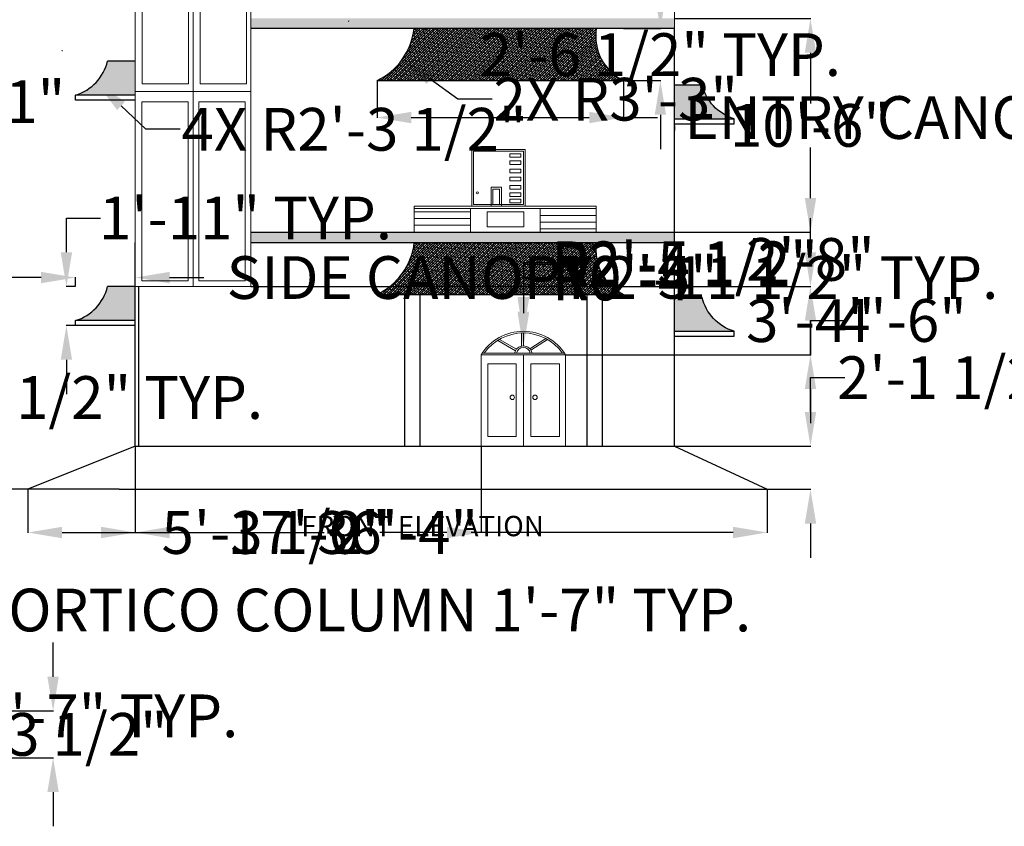
# Model space of a CAD drawing. Units: inches. Extents: x 28 to 3832, y 2 to 1709.
# Tile 5 of 7: x 2956 to 3536, y 863 to 1338. Entities that reach past the tile are written whole.
import ezdxf

# ---------------------------------------------------------------- set-up
doc = ezdxf.new("R2010")
doc.units = ezdxf.units.IN
doc.header["$MEASUREMENT"] = 0
for name, color, linetype, lineweight in [('A-ANNO-DIMS', 2, 'Continuous', 18), ('A-ANNO-TITL', 7, 'Continuous', 30), ('A-ELEV', 7, 'Continuous', 30), ('A-ELEV-DETL', 7, 'Continuous', 18), ('A-ELEV-OPEN', 4, 'Continuous', 18), ('A-ELEV-ROOF', 7, 'Continuous', 25)]:
    doc.layers.add(name, color=color, linetype=linetype, lineweight=lineweight)
doc.layers.add('A-ELEV-PATT', color=252, linetype='Continuous', lineweight=9, true_color=0x939598)
doc.layers.add('A-ROOF-PATT', color=30, linetype='Continuous', lineweight=9, true_color=0xf8991e)
doc.styles.get("Standard").update_dxf_attribs({"font": 'arial.ttf'})
doc.dimstyles.get("Standard").update_dxf_attribs({"dimtxt": 25.18, "dimasz": 20.18, "dimexe": 0.18, "dimexo": 0.0625, "dimgap": 0.09, "dimtad": 0, "dimtih": 1, "dimtoh": 1, "dimdec": 0, "dimzin": 0, "dimdsep": 46, "dimlunit": 3, "dimtxsty": 'Standard', "dimcen": 0.09, "dimadec": 0, "dimazin": 0, "dimtfac": 1, "dimtdec": 0, "dimtofl": 0, "dimtmove": 0, "dimatfit": 3, "dimfxl": 1, "dimtolj": 1, "dimtzin": 0, "dimarcsym": 0})
pattern_1 = [(45, (-138.4383, -52.9559), (-0.75130096, 0.75130096), []), (135, (-138.4383, -52.9559), (-2.25390287, 0.75130096), [2.65625, -1.59375])]

# ---------------------------------------------------------------- blocks, each defined once
blk = doc.blocks.new('SIDE-CANOPY-ELEV')
for p, q in [((35.31, 22.97), (18.94, 22.97)), ((0.06, 0), (0, 2.95)), ((0.06, 0), (0.12, 2.95)), ((35.31, 0), (0.06, 0)), ((35.31, 2.95), (0.12, 2.95))]:
    blk.add_line(p, q)
blk.add_arc((-7.77, 29.23), 27.43, 286.71454, 346.82691)
blk = doc.blocks.new('ENTRANCE-CANOPY-ELEV')
blk.add_line((0, 0), (145.27, 0))
for centre, radius, start, end in [((-16.67, 35.02), 38.79, 295.44798, 353.43172), ((157.97, 26.12), 29.04, 171.15568, 244.07718)]:
    blk.add_arc(centre, radius, start, end)
blk = doc.blocks.new('*D29')
at = {"layer": 'A-ANNO-DIMS', "color": 0, "lineweight": -2, "transparency": 16777216}
for p, q in [((2968.49, 1186.57), (2948.31, 1186.57)), ((2988.67, 1181.34), (2988.67, 1186.75)), ((3023.98, 1181.34), (3023.98, 1186.75)), ((3044.16, 1186.57), (3064.34, 1186.57))]:
    blk.add_line(p, q, dxfattribs=at)
at = {"layer": 'A-ANNO-DIMS', "color": 0, "transparency": 16777216}
for points in [[(2968.49, 1189.93), (2968.49, 1183.21), (2988.67, 1186.57)], [(3044.16, 1189.93), (3044.16, 1183.21), (3023.98, 1186.57)]]:
    blk.add_solid(points, dxfattribs=at)
at = {"layer": 'Defpoints', "color": 0, "transparency": 16777216}
for p in [(3023.98, 1186.57), (2988.67, 1181.27), (3023.98, 1181.27)]:
    blk.add_point(p, dxfattribs=at)
at = {"layer": 'A-ANNO-DIMS', "color": 0, "transparency": 16777216, "insert": (3305.33, 1186.57), "char_height": 25.18, "attachment_point": 5}
blk.add_mtext('\\A1;SIDE CANOPY 2\'-11 1/2" TYP.', dxfattribs=at)
blk = doc.blocks.new('*D30')
at = {"layer": 'A-ANNO-DIMS', "color": 0, "lineweight": -2, "transparency": 16777216}
for p, q in [((2983.37, 1201.45), (2983.37, 1221.63)), ((2983.37, 1221.63), (3003.55, 1221.63)), ((2988.6, 1181.27), (2983.19, 1181.27)), ((2988.6, 1158.3), (2983.19, 1158.3)), ((2983.37, 1138.12), (2983.37, 1117.94))]:
    blk.add_line(p, q, dxfattribs=at)
at = {"layer": 'A-ANNO-DIMS', "color": 0, "transparency": 16777216}
for points in [[(2980.01, 1201.45), (2986.73, 1201.45), (2983.37, 1181.27)], [(2980.01, 1138.12), (2986.73, 1138.12), (2983.37, 1158.3)]]:
    blk.add_solid(points, dxfattribs=at)
at = {"layer": 'Defpoints', "color": 0, "transparency": 16777216}
for p in [(2983.37, 1181.27), (2988.67, 1181.27), (2988.67, 1158.3)]:
    blk.add_point(p, dxfattribs=at)
at = {"layer": 'A-ANNO-DIMS', "color": 0, "transparency": 16777216, "insert": (3088.98, 1221.63), "char_height": 25.18, "attachment_point": 5}
blk.add_mtext('\\A1;1\'-11" TYP.', dxfattribs=at)
blk = doc.blocks.new('*D33')
at = {"layer": 'A-ANNO-DIMS', "color": 0, "lineweight": -2, "transparency": 16777216}
for p, q in [((2915.63, 1152.7), (2915.63, 1172.88)), ((2910.7, 1132.52), (2915.81, 1132.52)), ((2910.7, 1099.25), (2915.81, 1099.25)), ((2915.63, 1079.07), (2915.63, 1058.89))]:
    blk.add_line(p, q, dxfattribs=at)
at = {"layer": 'A-ANNO-DIMS', "color": 0, "transparency": 16777216}
for points in [[(2912.27, 1152.7), (2918.99, 1152.7), (2915.63, 1132.52)], [(2912.27, 1079.07), (2918.99, 1079.07), (2915.63, 1099.25)]]:
    blk.add_solid(points, dxfattribs=at)
at = {"layer": 'Defpoints', "color": 0, "transparency": 16777216}
for p in [(2910.64, 1132.52), (2910.64, 1099.25), (2915.63, 1099.25)]:
    blk.add_point(p, dxfattribs=at)
at = {"layer": 'A-ANNO-DIMS', "color": 0, "transparency": 16777216, "insert": (2915.63, 1115.88), "char_height": 25.18, "attachment_point": 5}
blk.add_mtext('\\A1;DOOR D2 2\'-9 1/2" TYP.', dxfattribs=at)
blk = doc.blocks.new('*D43')
at = {"layer": 'A-ANNO-DIMS', "color": 0, "lineweight": -2, "transparency": 16777216}
for p, q in [((2894.75, 970.5), (2894.75, 990.68)), ((2894.75, 990.68), (2914.93, 990.68)), ((2891.95, 950.32), (2894.93, 950.32)), ((2891.95, 931.2), (2894.93, 931.2)), ((2894.75, 911.02), (2894.75, 890.84))]:
    blk.add_line(p, q, dxfattribs=at)
at = {"layer": 'A-ANNO-DIMS', "color": 0, "transparency": 16777216}
for points in [[(2891.39, 970.5), (2898.12, 970.5), (2894.75, 950.32)], [(2891.39, 911.02), (2898.12, 911.02), (2894.75, 931.2)]]:
    blk.add_solid(points, dxfattribs=at)
at = {"layer": 'Defpoints', "color": 0, "transparency": 16777216}
for p in [(2891.88, 950.32), (2894.75, 950.32), (2891.88, 931.2)]:
    blk.add_point(p, dxfattribs=at)
at = {"layer": 'A-ANNO-DIMS', "color": 0, "transparency": 16777216, "insert": (3157.26, 990.68), "char_height": 25.18, "attachment_point": 5}
blk.add_mtext('\\A1;PORTICO COLUMN 1\'-7" TYP.', dxfattribs=at)
blk = doc.blocks.new('*D44')
at = {"layer": 'A-ANNO-DIMS', "color": 0, "lineweight": -2, "transparency": 16777216}
for p, q in [((2872.9, 931.14), (2872.9, 928.15)), ((2891.88, 931.14), (2891.88, 928.15)), ((2852.72, 928.33), (2832.54, 928.33)), ((2912.06, 928.33), (2932.24, 928.33))]:
    blk.add_line(p, q, dxfattribs=at)
at = {"layer": 'A-ANNO-DIMS', "color": 0, "transparency": 16777216}
for points in [[(2852.72, 931.69), (2852.72, 924.97), (2872.9, 928.33)], [(2912.06, 931.69), (2912.06, 924.97), (2891.88, 928.33)]]:
    blk.add_solid(points, dxfattribs=at)
at = {"layer": 'Defpoints', "color": 0, "transparency": 16777216}
for p in [(2872.9, 931.2), (2891.88, 931.2), (2891.88, 928.33)]:
    blk.add_point(p, dxfattribs=at)
at = {"layer": 'A-ANNO-DIMS', "color": 0, "transparency": 16777216, "insert": (3007.89, 928.33), "char_height": 25.18, "attachment_point": 5}
blk.add_mtext('\\A1;1\'-7" TYP.', dxfattribs=at)
blk = doc.blocks.new('*D45')
at = {"layer": 'A-ANNO-DIMS', "color": 0, "lineweight": -2, "transparency": 16777216}
for p, q in [((3166.51, 1302.58), (3166.51, 1280.67)), ((3311.78, 1302.58), (3311.78, 1280.67)), ((3186.69, 1280.85), (3291.6, 1280.85)), ((3311.78, 1280.85), (3331.96, 1280.85))]:
    blk.add_line(p, q, dxfattribs=at)
at = {"layer": 'A-ANNO-DIMS', "color": 0, "transparency": 16777216}
for points in [[(3186.69, 1284.21), (3186.69, 1277.49), (3166.51, 1280.85)], [(3291.6, 1284.21), (3291.6, 1277.49), (3311.78, 1280.85)]]:
    blk.add_solid(points, dxfattribs=at)
at = {"layer": 'Defpoints', "color": 0, "transparency": 16777216}
for p in [(3166.51, 1302.64), (3311.78, 1302.64), (3311.78, 1280.85)]:
    blk.add_point(p, dxfattribs=at)
at = {"layer": 'A-ANNO-DIMS', "color": 0, "transparency": 16777216, "insert": (3590.91, 1280.85), "char_height": 25.18, "attachment_point": 5}
blk.add_mtext('\\A1;ENTRY CANOPY 12\'-1 1/2" TYP.', dxfattribs=at)
blk = doc.blocks.new('*D46')
at = {"layer": 'A-ANNO-DIMS', "color": 0, "lineweight": -2, "transparency": 16777216}
for p, q in [((3333.57, 1353.41), (3333.57, 1373.59)), ((3311.84, 1333.23), (3333.75, 1333.23)), ((3311.84, 1302.64), (3333.75, 1302.64)), ((3333.57, 1282.46), (3333.57, 1262.28))]:
    blk.add_line(p, q, dxfattribs=at)
at = {"layer": 'A-ANNO-DIMS', "color": 0, "transparency": 16777216}
for points in [[(3330.21, 1353.41), (3336.94, 1353.41), (3333.57, 1333.23)], [(3330.21, 1282.46), (3336.94, 1282.46), (3333.57, 1302.64)]]:
    blk.add_solid(points, dxfattribs=at)
at = {"layer": 'Defpoints', "color": 0, "transparency": 16777216}
for p in [(3311.78, 1333.23), (3333.57, 1333.23), (3311.78, 1302.64)]:
    blk.add_point(p, dxfattribs=at)
at = {"layer": 'A-ANNO-DIMS', "color": 0, "transparency": 16777216, "insert": (3333.57, 1317.94), "char_height": 25.18, "attachment_point": 5}
blk.add_mtext('\\A1;2\'-6 1/2" TYP.', dxfattribs=at)
blk = doc.blocks.new('*D52')
at = {"layer": 'A-ANNO-DIMS', "color": 0, "lineweight": -2, "transparency": 16777216}
for p, q in [((2975.53, 951.38), (2975.53, 971.56)), ((2891.95, 931.2), (2975.71, 931.2)), ((2906.74, 903.61), (2975.71, 903.61)), ((2975.53, 883.43), (2975.53, 863.25))]:
    blk.add_line(p, q, dxfattribs=at)
at = {"layer": 'A-ANNO-DIMS', "color": 0, "transparency": 16777216}
for points in [[(2972.16, 951.38), (2978.89, 951.38), (2975.53, 931.2)], [(2972.16, 883.43), (2978.89, 883.43), (2975.53, 903.61)]]:
    blk.add_solid(points, dxfattribs=at)
at = {"layer": 'Defpoints', "color": 0, "transparency": 16777216}
for p in [(2891.88, 931.2), (2975.53, 931.2), (2906.67, 903.61)]:
    blk.add_point(p, dxfattribs=at)
at = {"layer": 'A-ANNO-DIMS', "color": 0, "transparency": 16777216, "insert": (2975.53, 917.41), "char_height": 25.18, "attachment_point": 5}
blk.add_mtext('\\A1;2\'-3 1/2"', dxfattribs=at)
blk = doc.blocks.new('*D53')
at = {"layer": 'A-ANNO-DIMS', "color": 0, "lineweight": -2, "transparency": 16777216}
for p, q in [((2960.67, 1061.73), (2960.67, 1036.17)), ((3396.62, 1061.73), (3396.62, 1036.17)), ((2980.85, 1036.35), (3135.31, 1036.35)), ((3376.44, 1036.35), (3221.98, 1036.35))]:
    blk.add_line(p, q, dxfattribs=at)
at = {"layer": 'A-ANNO-DIMS', "color": 0, "transparency": 16777216}
for points in [[(2980.85, 1039.71), (2980.85, 1032.98), (2960.67, 1036.35)], [(3376.44, 1039.71), (3376.44, 1032.98), (3396.62, 1036.35)]]:
    blk.add_solid(points, dxfattribs=at)
at = {"layer": 'Defpoints', "color": 0, "transparency": 16777216}
for p in [(2960.67, 1061.8), (3396.62, 1061.8), (3396.62, 1036.35)]:
    blk.add_point(p, dxfattribs=at)
at = {"layer": 'A-ANNO-DIMS', "color": 0, "transparency": 16777216, "insert": (3178.65, 1036.35), "char_height": 25.18, "attachment_point": 5}
blk.add_mtext('\\A1;36\'-4"', dxfattribs=at)
blk = doc.blocks.new('*D54')
at = {"layer": 'A-ANNO-DIMS', "color": 0, "lineweight": -2, "transparency": 16777216}
for p, q in [((3022.59, 1518.63), (2935.04, 1518.63)), ((2935.22, 1498.45), (2935.22, 1303.17)), ((2935.22, 1081.98), (2935.22, 1277.26)), ((2960.61, 1061.8), (2935.04, 1061.8))]:
    blk.add_line(p, q, dxfattribs=at)
at = {"layer": 'A-ANNO-DIMS', "color": 0, "transparency": 16777216}
for points in [[(2931.86, 1498.45), (2938.58, 1498.45), (2935.22, 1518.63)], [(2931.86, 1081.98), (2938.58, 1081.98), (2935.22, 1061.8)]]:
    blk.add_solid(points, dxfattribs=at)
at = {"layer": 'Defpoints', "color": 0, "transparency": 16777216}
for p in [(2935.22, 1518.63), (3022.65, 1518.63), (2960.67, 1061.8)]:
    blk.add_point(p, dxfattribs=at)
at = {"layer": 'A-ANNO-DIMS', "color": 0, "transparency": 16777216, "insert": (2935.22, 1290.21), "char_height": 25.18, "attachment_point": 5}
blk.add_mtext('\\A1;38\'-1"', dxfattribs=at)
blk = doc.blocks.new('*D57')
at = {"layer": 'A-ANNO-DIMS', "color": 0, "lineweight": -2, "transparency": 16777216}
for p, q in [((3422.07, 1107.41), (3422.07, 1127.59)), ((3422.07, 1127.59), (3442.25, 1127.59)), ((3341.88, 1087.23), (3422.25, 1087.23)), ((3396.68, 1061.8), (3422.25, 1061.8)), ((3422.07, 1041.62), (3422.07, 1021.44))]:
    blk.add_line(p, q, dxfattribs=at)
at = {"layer": 'A-ANNO-DIMS', "color": 0, "transparency": 16777216}
for points in [[(3418.71, 1107.41), (3425.43, 1107.41), (3422.07, 1087.23)], [(3418.71, 1041.62), (3425.43, 1041.62), (3422.07, 1061.8)]]:
    blk.add_solid(points, dxfattribs=at)
at = {"layer": 'Defpoints', "color": 0, "transparency": 16777216}
for p in [(3341.81, 1087.23), (3422.07, 1087.23), (3396.62, 1061.8)]:
    blk.add_point(p, dxfattribs=at)
at = {"layer": 'A-ANNO-DIMS', "color": 0, "transparency": 16777216, "insert": (3505.36, 1127.59), "char_height": 25.18, "attachment_point": 5}
blk.add_mtext('\\A1;2\'-1 1/2"', dxfattribs=at)
blk = doc.blocks.new('*D58')
at = {"layer": 'A-ANNO-DIMS', "color": 0, "lineweight": -2, "transparency": 16777216}
for p, q in [((3422.07, 1141.09), (3422.07, 1161.27)), ((3422.07, 1161.27), (3442.25, 1161.27)), ((3277.74, 1141.09), (3422.25, 1141.09)), ((3422.07, 1107.41), (3422.07, 1120.91)), ((3341.88, 1087.23), (3422.25, 1087.23))]:
    blk.add_line(p, q, dxfattribs=at)
at = {"layer": 'A-ANNO-DIMS', "color": 0, "transparency": 16777216}
for points in [[(3418.71, 1120.91), (3425.43, 1120.91), (3422.07, 1141.09)], [(3418.71, 1107.41), (3425.43, 1107.41), (3422.07, 1087.23)]]:
    blk.add_solid(points, dxfattribs=at)
at = {"layer": 'Defpoints', "color": 0, "transparency": 16777216}
for p in [(3277.68, 1141.09), (3422.07, 1141.09), (3341.81, 1087.23)]:
    blk.add_point(p, dxfattribs=at)
at = {"layer": 'A-ANNO-DIMS', "color": 0, "transparency": 16777216, "insert": (3476.31, 1161.27), "char_height": 25.18, "attachment_point": 5}
blk.add_mtext('\\A1;4\'-6"', dxfattribs=at)
blk = doc.blocks.new('*D59')
at = {"layer": 'A-ANNO-DIMS', "color": 0, "lineweight": -2, "transparency": 16777216}
for p, q in [((3422.07, 1201.45), (3422.07, 1221.63)), ((3092.19, 1181.27), (3422.25, 1181.27)), ((3277.74, 1141.09), (3422.25, 1141.09)), ((3422.07, 1120.91), (3422.07, 1100.73))]:
    blk.add_line(p, q, dxfattribs=at)
at = {"layer": 'A-ANNO-DIMS', "color": 0, "transparency": 16777216}
for points in [[(3418.71, 1201.45), (3425.43, 1201.45), (3422.07, 1181.27)], [(3418.71, 1120.91), (3425.43, 1120.91), (3422.07, 1141.09)]]:
    blk.add_solid(points, dxfattribs=at)
at = {"layer": 'Defpoints', "color": 0, "transparency": 16777216}
for p in [(3092.13, 1181.27), (3422.07, 1181.27), (3277.68, 1141.09)]:
    blk.add_point(p, dxfattribs=at)
at = {"layer": 'A-ANNO-DIMS', "color": 0, "transparency": 16777216, "insert": (3422.07, 1161.18), "char_height": 25.18, "attachment_point": 5}
blk.add_mtext('\\A1;3\'-4"', dxfattribs=at)
blk = doc.blocks.new('*D60')
at = {"layer": 'A-ANNO-DIMS', "color": 0, "lineweight": -2, "transparency": 16777216}
for p, q in [((3422.07, 1233.41), (3422.07, 1253.59)), ((3341.88, 1213.23), (3422.25, 1213.23)), ((3092.19, 1181.27), (3422.25, 1181.27)), ((3422.07, 1161.09), (3422.07, 1140.91))]:
    blk.add_line(p, q, dxfattribs=at)
at = {"layer": 'A-ANNO-DIMS', "color": 0, "transparency": 16777216}
for points in [[(3418.71, 1233.41), (3425.43, 1233.41), (3422.07, 1213.23)], [(3418.71, 1161.09), (3425.43, 1161.09), (3422.07, 1181.27)]]:
    blk.add_solid(points, dxfattribs=at)
at = {"layer": 'Defpoints', "color": 0, "transparency": 16777216}
for p in [(3341.81, 1213.23), (3422.07, 1213.23), (3092.13, 1181.27)]:
    blk.add_point(p, dxfattribs=at)
at = {"layer": 'A-ANNO-DIMS', "color": 0, "transparency": 16777216, "insert": (3422.07, 1197.25), "char_height": 25.18, "attachment_point": 5}
blk.add_mtext('\\A1;2\'-8"', dxfattribs=at)
blk = doc.blocks.new('*D61')
at = {"layer": 'A-ANNO-DIMS', "color": 0, "lineweight": -2, "transparency": 16777216}
for p, q in [((3341.88, 1339.23), (3422.25, 1339.23)), ((3422.07, 1319.05), (3422.07, 1289.18)), ((3422.07, 1233.41), (3422.07, 1263.28)), ((3341.88, 1213.23), (3422.25, 1213.23))]:
    blk.add_line(p, q, dxfattribs=at)
at = {"layer": 'A-ANNO-DIMS', "color": 0, "transparency": 16777216}
for points in [[(3418.71, 1319.05), (3425.43, 1319.05), (3422.07, 1339.23)], [(3418.71, 1233.41), (3425.43, 1233.41), (3422.07, 1213.23)]]:
    blk.add_solid(points, dxfattribs=at)
at = {"layer": 'Defpoints', "color": 0, "transparency": 16777216}
for p in [(3341.81, 1339.23), (3422.07, 1339.23), (3341.81, 1213.23)]:
    blk.add_point(p, dxfattribs=at)
at = {"layer": 'A-ANNO-DIMS', "color": 0, "transparency": 16777216, "insert": (3422.07, 1276.23), "char_height": 25.18, "attachment_point": 5}
blk.add_mtext('\\A1;10\'-6"', dxfattribs=at)
blk = doc.blocks.new('*D65')
at = {"layer": 'A-ANNO-DIMS', "color": 0, "lineweight": -2, "transparency": 16777216}
for p, q in [((3023.98, 1087.17), (3023.98, 1036.17)), ((2960.67, 1061.73), (2960.67, 1036.17)), ((2980.85, 1036.35), (3003.8, 1036.35)), ((3023.98, 1036.35), (3044.16, 1036.35))]:
    blk.add_line(p, q, dxfattribs=at)
at = {"layer": 'A-ANNO-DIMS', "color": 0, "transparency": 16777216}
for points in [[(2980.85, 1039.71), (2980.85, 1032.98), (2960.67, 1036.35)], [(3003.8, 1039.71), (3003.8, 1032.98), (3023.98, 1036.35)]]:
    blk.add_solid(points, dxfattribs=at)
at = {"layer": 'Defpoints', "color": 0, "transparency": 16777216}
for p in [(3023.98, 1087.23), (2960.67, 1061.8), (3023.98, 1036.35)]:
    blk.add_point(p, dxfattribs=at)
at = {"layer": 'A-ANNO-DIMS', "color": 0, "transparency": 16777216, "insert": (3107.05, 1036.35), "char_height": 25.18, "attachment_point": 5}
blk.add_mtext('\\A1;5\'-3 1/2"', dxfattribs=at)
blk = doc.blocks.new('*D66')
at = {"layer": 'A-ANNO-DIMS', "color": 0, "lineweight": -2, "transparency": 16777216}
for p, q in [((3023.98, 1087.17), (3023.98, 1036.17)), ((3227.89, 1087.17), (3227.89, 1036.17)), ((3044.16, 1036.35), (3083.78, 1036.35)), ((3207.71, 1036.35), (3168.09, 1036.35))]:
    blk.add_line(p, q, dxfattribs=at)
at = {"layer": 'A-ANNO-DIMS', "color": 0, "transparency": 16777216}
for points in [[(3044.16, 1039.71), (3044.16, 1032.98), (3023.98, 1036.35)], [(3207.71, 1039.71), (3207.71, 1032.98), (3227.89, 1036.35)]]:
    blk.add_solid(points, dxfattribs=at)
at = {"layer": 'Defpoints', "color": 0, "transparency": 16777216}
for p in [(3023.98, 1087.23), (3227.89, 1087.23), (3227.89, 1036.35)]:
    blk.add_point(p, dxfattribs=at)
at = {"layer": 'A-ANNO-DIMS', "color": 0, "transparency": 16777216, "insert": (3125.93, 1036.35), "char_height": 25.18, "attachment_point": 5}
blk.add_mtext('\\A1;17\'-0"', dxfattribs=at)
blk = doc.blocks.new('*D76')
at = {"layer": 'A-ANNO-DIMS', "color": 0, "lineweight": -2, "transparency": 16777216}
for p, q in [((3272.96, 1195.27), (3252.78, 1195.27)), ((3252.78, 1195.27), (3252.78, 1175.09)), ((3252.69, 1125.57), (3252.87, 1125.57)), ((3252.78, 1125.48), (3252.78, 1125.66))]:
    blk.add_line(p, q, dxfattribs=at)
at = {"layer": 'A-ANNO-DIMS', "color": 0, "transparency": 16777216}
blk.add_solid([(3249.42, 1175.09), (3256.15, 1175.09), (3252.78, 1154.91)], dxfattribs=at)
at = {"layer": 'Defpoints', "color": 0, "transparency": 16777216}
for p in [(3252.78, 1154.91), (3252.78, 1125.57)]:
    blk.add_point(p, dxfattribs=at)
at = {"layer": 'A-ANNO-DIMS', "color": 0, "transparency": 16777216, "insert": (3347.91, 1195.27), "char_height": 25.18, "attachment_point": 5}
blk.add_mtext('\\A1;R2\'-5 1/2"', dxfattribs=at)
blk = doc.blocks.new('*D77')
at = {"layer": 'A-ANNO-DIMS', "color": 0, "lineweight": -2, "transparency": 16777216}
for p, q in [((3272.96, 1194.27), (3252.78, 1194.27)), ((3252.78, 1194.27), (3252.78, 1174.09)), ((3252.69, 1125.57), (3252.87, 1125.57)), ((3252.78, 1125.48), (3252.78, 1125.66))]:
    blk.add_line(p, q, dxfattribs=at)
at = {"layer": 'A-ANNO-DIMS', "color": 0, "transparency": 16777216}
blk.add_solid([(3249.42, 1174.09), (3256.15, 1174.09), (3252.78, 1153.91)], dxfattribs=at)
at = {"layer": 'Defpoints', "color": 0, "transparency": 16777216}
for p in [(3252.78, 1153.91), (3252.78, 1125.57)]:
    blk.add_point(p, dxfattribs=at)
at = {"layer": 'A-ANNO-DIMS', "color": 0, "transparency": 16777216, "insert": (3347.91, 1194.27), "char_height": 25.18, "attachment_point": 5}
blk.add_mtext('\\A1;R2\'-4 1/2"', dxfattribs=at)
blk = doc.blocks.new('*D78')
at = {"layer": 'A-ANNO-DIMS', "color": 0, "lineweight": -2, "transparency": 16777216}
for p, q in [((3252.79, 1186.68), (3252.78, 1166.5)), ((3272.97, 1186.68), (3252.79, 1186.68)), ((3252.69, 1141.09), (3252.87, 1141.09)), ((3252.78, 1141), (3252.78, 1141.18))]:
    blk.add_line(p, q, dxfattribs=at)
at = {"layer": 'A-ANNO-DIMS', "color": 0, "transparency": 16777216}
blk.add_solid([(3249.42, 1166.5), (3256.15, 1166.5), (3252.78, 1146.32)], dxfattribs=at)
at = {"layer": 'Defpoints', "color": 0, "transparency": 16777216}
for p in [(3252.78, 1146.32), (3252.78, 1141.09)]:
    blk.add_point(p, dxfattribs=at)
at = {"layer": 'A-ANNO-DIMS', "color": 0, "transparency": 16777216, "insert": (3318.57, 1186.68), "char_height": 25.18, "attachment_point": 5}
blk.add_mtext('\\A1;R0\'-5"', dxfattribs=at)
blk = doc.blocks.new('*D79')
at = {"layer": 'A-ANNO-DIMS', "color": 0, "lineweight": -2, "transparency": 16777216}
for p, q in [((3252.79, 1185.68), (3252.78, 1165.5)), ((3272.97, 1185.68), (3252.79, 1185.68)), ((3252.69, 1141.09), (3252.87, 1141.09)), ((3252.78, 1141), (3252.78, 1141.18))]:
    blk.add_line(p, q, dxfattribs=at)
at = {"layer": 'A-ANNO-DIMS', "color": 0, "transparency": 16777216}
blk.add_solid([(3249.42, 1165.5), (3256.15, 1165.5), (3252.78, 1145.32)], dxfattribs=at)
at = {"layer": 'Defpoints', "color": 0, "transparency": 16777216}
for p in [(3252.78, 1145.32), (3252.78, 1141.09)]:
    blk.add_point(p, dxfattribs=at)
at = {"layer": 'A-ANNO-DIMS', "color": 0, "transparency": 16777216, "insert": (3318.57, 1185.68), "char_height": 25.18, "attachment_point": 5}
blk.add_mtext('\\A1;R0\'-4"', dxfattribs=at)
blk = doc.blocks.new('*D80')
at = {"layer": 'A-ANNO-DIMS', "color": 0, "lineweight": -2, "transparency": 16777216}
for p, q in [((3149.75, 1337.67), (3149.93, 1337.67)), ((3149.84, 1337.58), (3149.84, 1337.76)), ((3214.23, 1291.64), (3197.81, 1303.37)), ((3234.41, 1291.64), (3214.23, 1291.64))]:
    blk.add_line(p, q, dxfattribs=at)
at = {"layer": 'A-ANNO-DIMS', "color": 0, "transparency": 16777216}
blk.add_solid([(3199.77, 1306.11), (3195.85, 1300.64), (3181.39, 1315.11)], dxfattribs=at)
at = {"layer": 'Defpoints', "color": 0, "transparency": 16777216}
for p in [(3149.84, 1337.67), (3181.39, 1315.11)]:
    blk.add_point(p, dxfattribs=at)
at = {"layer": 'A-ANNO-DIMS', "color": 0, "transparency": 16777216, "insert": (3307.28, 1291.64), "char_height": 25.18, "attachment_point": 5}
blk.add_mtext('\\A1;2X R3\'-3"', dxfattribs=at)
blk = doc.blocks.new('*D81')
at = {"layer": 'A-ANNO-DIMS', "color": 0, "lineweight": -2, "transparency": 16777216}
for p, q in [((2980.81, 1320.37), (2980.99, 1320.37)), ((2980.9, 1320.28), (2980.9, 1320.46)), ((3030.29, 1273.94), (3015.59, 1287.76)), ((3050.47, 1273.94), (3030.29, 1273.94))]:
    blk.add_line(p, q, dxfattribs=at)
at = {"layer": 'A-ANNO-DIMS', "color": 0, "transparency": 16777216}
blk.add_solid([(3017.89, 1290.21), (3013.28, 1285.31), (3000.88, 1301.58)], dxfattribs=at)
at = {"layer": 'Defpoints', "color": 0, "transparency": 16777216}
for p in [(2980.9, 1320.37), (3000.88, 1301.58)]:
    blk.add_point(p, dxfattribs=at)
at = {"layer": 'A-ANNO-DIMS', "color": 0, "transparency": 16777216, "insert": (3152.97, 1273.94), "char_height": 25.18, "attachment_point": 5}
blk.add_mtext('\\A1;4X R2\'-3 1/2"', dxfattribs=at)

msp = doc.modelspace()

# ---------------------------------------------------------------- hatches: boundary and pattern name
at = {"layer": 'A-ELEV-PATT'}
h = msp.add_hatch(color=256, dxfattribs=at)
h.dxf.hatch_style = 1
h.paths.add_polyline_path([(3341.81, 1339.23), (3092.13, 1339.23), (3092.13, 1333.23), (3341.81, 1333.23)])
h.paths.add_polyline_path([(3341.81, 1213.23), (3092.13, 1213.23), (3092.13, 1207.23), (3341.81, 1207.23)])
at = {"layer": 'A-ROOF-PATT'}
h = msp.add_hatch(dxfattribs=at)
h.set_pattern_fill('ANSI38', color=256, scale=8.5)
h.set_pattern_definition([(45, (-138.5602, 73.0441), (-0.75130096, 0.75130096), []), (135, (-138.5602, 73.0441), (-2.25390287, 0.75130096), [2.65625, -1.59375])])
h.paths.add_polyline_path([(3295.78, 1333.23), (3188.37, 1333.23, -0.258542), (3166.51, 1302.64), (3311.78, 1302.64, -0.329371)])
h = msp.add_hatch(dxfattribs=at)
h.set_pattern_fill('ANSI38', color=256, scale=8.5)
h.set_pattern_definition(pattern_1)
h.paths.add_polyline_path([(3023.98, 1314.12), (3007.61, 1314.12, -0.268475), (2988.79, 1294.1), (3023.98, 1294.1)])
h.paths.add_polyline_path([(3023.98, 1161.25), (3023.98, 1181.27), (3007.61, 1181.27, -0.268475), (2988.79, 1161.25)])
h.paths.add_polyline_path([(3358.18, 1300.2), (3341.81, 1300.2), (3341.81, 1280.17), (3377, 1280.17, -0.268475)])
h.paths.add_polyline_path([(3341.81, 1174.96), (3341.81, 1154.94), (3377, 1154.94, -0.268475), (3358.18, 1174.96)])
h = msp.add_hatch(dxfattribs=at)
h.set_pattern_fill('ANSI38', color=256, scale=8.5)
h.set_pattern_definition(pattern_1)
h.paths.add_polyline_path([(3295.9, 1207.23), (3188.5, 1207.23, -0.258542), (3166.63, 1176.64), (3311.9, 1176.64, -0.329371)])

# ---------------------------------------------------------------- linework, layer by layer
at = {"layer": 'A-ELEV'}
for p, q in [((3341.81, 1333.23), (3092.13, 1333.23)), ((3341.81, 1213.23), (3341.81, 1333.23)), ((3341.81, 1296.17), (3341.81, 1296.17)), ((3341.81, 1276.14), (3341.81, 1273.19)), ((3341.81, 1087.23), (3341.81, 1273.19)), ((3092.13, 1213.23), (3341.81, 1213.23)), ((3023.98, 1087.23), (3023.98, 1207.23)), ((3092.13, 1207.23), (3341.81, 1207.23)), ((3025.98, 1087.23), (3025.98, 1181.27)), ((3182.89, 1087.23), (3182.89, 1176.64)), ((3191.89, 1087.23), (3191.89, 1176.64)), ((3290.47, 1087.23), (3290.47, 1176.64)), ((3299.47, 1087.23), (3299.47, 1176.64)), ((3023.98, 1087.23), (2960.67, 1061.8)), ((3023.98, 1087.23), (3341.81, 1087.23)), ((3341.81, 1087.23), (3396.62, 1061.8)), ((3014.42, 1061.8), (2960.67, 1061.8)), ((3014.42, 1061.8), (3374.42, 1061.8)), ((3374.42, 1061.8), (3396.62, 1061.8))]:
    msp.add_line(p, q, dxfattribs=at)
msp.add_lwpolyline([(3188.5, 1207.23), (3295.78, 1207.23)], dxfattribs=at)
at = {"layer": 'A-ELEV-DETL'}
for p, q in [((3341.81, 1385.25), (3341.81, 1333.23)), ((3188.5, 1228.62), (3295.78, 1228.62)), ((3221.66, 1227.2), (3188.5, 1227.2)), ((3221.66, 1225.36), (3188.5, 1225.36)), ((3262.76, 1227.2), (3295.78, 1227.2)), ((3221.66, 1221.36), (3188.5, 1221.36)), ((3262.76, 1223.2), (3295.78, 1223.2)), ((3262.76, 1219.2), (3295.78, 1219.2)), ((3221.66, 1217.36), (3188.5, 1217.36)), ((3221.66, 1213.36), (3188.5, 1213.36)), ((3262.76, 1215.2), (3295.78, 1215.2))]:
    msp.add_line(p, q, dxfattribs=at)
for points in [[(3188.5, 1228.62), (3188.5, 1213.23)], [(3221.66, 1213.23), (3221.66, 1227.2), (3262.76, 1227.2), (3262.76, 1213.23)], [(3295.78, 1213.23), (3295.78, 1228.62)]]:
    msp.add_lwpolyline(points, dxfattribs=at)
msp.add_lwpolyline([(3231.48, 1225.22), (3253.01, 1225.22), (3253.01, 1216.39), (3231.48, 1216.39)], close=True, dxfattribs=at)
at = {"layer": 'A-ELEV-OPEN'}
for p, q in [((3058.05, 1411.18), (3058.05, 1181.27)), ((3023.98, 1296.23), (3092.13, 1296.23)), ((3248.17, 1143.45), (3237.67, 1149.54)), ((3248.67, 1144.32), (3238.65, 1150.13)), ((3251.78, 1146.32), (3251.78, 1153.91)), ((3252.78, 1146.32), (3252.78, 1153.91)), ((3256.63, 1144.63), (3265.96, 1150.66)), ((3257.17, 1143.79), (3266.95, 1150.11)), ((3252.78, 1141.09), (3252.78, 1087.23))]:
    msp.add_line(p, q, dxfattribs=at)
for points in [[(3023.98, 1181.27), (3092.13, 1181.27), (3092.13, 1411.18), (3023.98, 1411.18)], [(3028.11, 1406.28), (3055.43, 1406.28), (3055.43, 1300.77), (3028.11, 1300.77)], [(3062.25, 1406.28), (3089.57, 1406.28), (3089.57, 1300.77), (3062.25, 1300.77)], [(3027.78, 1290.2), (3055.1, 1290.2), (3055.1, 1184.69), (3027.78, 1184.69)], [(3061.45, 1290.2), (3088.77, 1290.2), (3088.77, 1184.69), (3061.45, 1184.69)], [(3222.39, 1228.62), (3253.79, 1228.62), (3253.79, 1261.94), (3222.39, 1261.94)], [(3223.39, 1229.62), (3252.79, 1229.62), (3252.79, 1260.94), (3223.39, 1260.94)], [(3244.83, 1259.54), (3251.2, 1259.54), (3251.2, 1257.41), (3244.83, 1257.41)], [(3244.83, 1255.37), (3251.2, 1255.37), (3251.2, 1253.24), (3244.83, 1253.24)], [(3244.83, 1250.44), (3251.2, 1250.44), (3251.2, 1248.31), (3244.83, 1248.31)], [(3244.83, 1245.66), (3251.2, 1245.66), (3251.2, 1243.53), (3244.83, 1243.53)], [(3233.77, 1228.62), (3239.81, 1228.62), (3239.81, 1239.73), (3233.77, 1239.73)], [(3234.77, 1229.62), (3238.81, 1229.62), (3238.81, 1238.73), (3234.77, 1238.73)], [(3244.83, 1240.8), (3251.2, 1240.8), (3251.2, 1238.68), (3244.83, 1238.68)], [(3244.83, 1236.52), (3251.2, 1236.52), (3251.2, 1234.4), (3244.83, 1234.4)], [(3244.83, 1232.77), (3251.2, 1232.77), (3251.2, 1230.65), (3244.83, 1230.65)], [(3227.89, 1087.23), (3277.68, 1087.23), (3277.68, 1141.09), (3227.89, 1141.09)], [(3231.77, 1135.65), (3248.54, 1135.65), (3248.54, 1092.92), (3231.77, 1092.92)], [(3257.29, 1135.65), (3274.06, 1135.65), (3274.06, 1092.92), (3257.29, 1092.92)]]:
    msp.add_lwpolyline(points, close=True, dxfattribs=at)
msp.add_lwpolyline([(3277.02, 1142.09), (3228.54, 1142.09)], dxfattribs=at)
for centre, radius in [((3225.72, 1236.49), 0.68), ((3246.25, 1115.97), 1.31), ((3259.67, 1115.97), 1.31)]:
    msp.add_circle(centre, radius, dxfattribs=at)
for centre, radius, start, end in [((3252.78, 1125.57), 29.34, 31.95292, 148.04708), ((3252.78, 1125.57), 28.34, 35.67503, 144.32497), ((3252.78, 1141.09), 5.22, 11.03824, 168.96176), ((3252.78, 1141.09), 4.22, 13.69796, 166.30204)]:
    msp.add_arc(centre, radius, start, end, dxfattribs=at)

# ---------------------------------------------------------------- block references
at = {"layer": 'A-ELEV-ROOF'}
for name, p in [('ENTRANCE-CANOPY-ELEV', (3166.51, 1302.64)), ('SIDE-CANOPY-ELEV', (2988.67, 1291.14)), ('ENTRANCE-CANOPY-ELEV', (3166.63, 1176.64)), ('SIDE-CANOPY-ELEV', (2988.67, 1158.3))]:
    msp.add_blockref(name, p, dxfattribs=at)
at = {"layer": 'A-ELEV-ROOF', "extrusion": (0, 0, -1), "zscale": -1}
for p in [(-3377.12, 1277.22), (-3377.12, 1151.99)]:
    msp.add_blockref('SIDE-CANOPY-ELEV', p, dxfattribs=at)

# ---------------------------------------------------------------- texts
at = {"layer": 'A-ANNO-TITL', "insert": (3121.87, 1046.16), "char_height": 12, "attachment_point": 1}
msp.add_mtext_dynamic_manual_height_columns('FRONT ELEVATION', width=231.9537, gutter_width=1, heights=[0], dxfattribs=at)

# ---------------------------------------------------------------- dimensions: what is measured, and where the dimension line sits
at = {"layer": 'A-ANNO-DIMS'}
for base, p1, p2, picture, middle in [((2935.22, 1518.63), (2960.67, 1061.8), (3022.65, 1518.63), '*D54', (2935.22, 1290.21)), ((3422.07, 1339.23), (3341.81, 1213.23), (3341.81, 1339.23), '*D61', (3422.07, 1276.23)), ((3422.07, 1213.23), (3092.13, 1181.27), (3341.81, 1213.23), '*D60', (3422.07, 1197.25)), ((3422.07, 1181.27), (3277.68, 1141.09), (3092.13, 1181.27), '*D59', (3422.07, 1161.18)), ((3422.07, 1141.09), (3341.81, 1087.23), (3277.68, 1141.09), '*D58', (3476.31, 1161.27)), ((3422.07, 1087.23), (3396.62, 1061.8), (3341.81, 1087.23), '*D57', (3505.36, 1127.59)), ((2975.53, 931.2), (2906.67, 903.61), (2891.88, 931.2), '*D52', (2975.53, 917.41))]:
    dim = msp.add_linear_dim(base=base, p1=p1, p2=p2, angle=90, dimstyle='Standard', override={"dimdec": 1, "dimlfac": 1, "dimrnd": 0, "dimzin": 1, "dimdsep": 46, "dimlunit": 4, "dimfrac": 2}, dxfattribs=at)
    dim.commit()
    dim.dimension.update_dxf_attribs({"geometry": picture, "text_midpoint": middle})
for base, p1, p2, text, picture, middle in [((3311.78, 1280.85), (3166.51, 1302.64), (3311.78, 1302.64), 'ENTRY CANOPY <> TYP.', '*D45', (3590.91, 1280.85)), ((3023.98, 1186.57), (2988.67, 1181.27), (3023.98, 1181.27), 'SIDE CANOPY <> TYP.', '*D29', (3305.33, 1186.57)), ((2891.88, 928.33), (2872.9, 931.2), (2891.88, 931.2), '<> TYP.', '*D44', (3007.89, 928.33))]:
    dim = msp.add_linear_dim(base=base, p1=p1, p2=p2, text=text, dimstyle='Standard', override={"dimdec": 1, "dimlfac": 1, "dimrnd": 0, "dimzin": 1, "dimdsep": 46, "dimlunit": 4, "dimfrac": 2}, dxfattribs=at)
    dim.commit()
    dim.dimension.update_dxf_attribs({"geometry": picture, "text_midpoint": middle})
for base, p1, p2, angle, text, picture, middle in [((3333.57, 1333.23), (3311.78, 1302.64), (3311.78, 1333.23), 90, '<> TYP.', '*D46', (3333.57, 1317.94)), ((2983.37, 1181.27), (2988.67, 1158.3), (2988.67, 1181.27), 90, '<> TYP.', '*D30', (3088.98, 1221.63)), ((2915.63, 1099.25), (2910.64, 1132.52), (2910.64, 1099.25), 270, 'DOOR D2 <> TYP.', '*D33', (2915.63, 1115.88)), ((2894.75, 950.32), (2891.88, 931.2), (2891.88, 950.32), 90, 'PORTICO COLUMN <> TYP.', '*D43', (3157.26, 990.68))]:
    dim = msp.add_linear_dim(base=base, p1=p1, p2=p2, angle=angle, text=text, dimstyle='Standard', override={"dimdec": 1, "dimlfac": 1, "dimrnd": 0, "dimzin": 1, "dimdsep": 46, "dimlunit": 4, "dimfrac": 2}, dxfattribs=at)
    dim.commit()
    dim.dimension.update_dxf_attribs({"geometry": picture, "text_midpoint": middle})
for center, mpoint, text, picture, middle in [((3149.84, 1337.67), (3181.39, 1315.11), '2X <>', '*D80', (3307.28, 1291.64)), ((2980.9, 1320.37), (3000.88, 1301.58), '4X <>', '*D81', (3152.97, 1273.94))]:
    dim = msp.add_radius_dim(center=center, mpoint=mpoint, text=text, dimstyle='Standard', override={"dimdec": 1, "dimlfac": 1, "dimrnd": 0, "dimzin": 1, "dimdsep": 46, "dimlunit": 4, "dimfrac": 2}, dxfattribs=at)
    dim.commit()
    dim.dimension.update_dxf_attribs({"geometry": picture, "text_midpoint": middle})
for center, mpoint, picture, middle in [((3252.78, 1125.57), (3252.78, 1154.91), '*D76', (3347.91, 1195.27)), ((3252.78, 1125.57), (3252.78, 1153.91), '*D77', (3347.91, 1194.27)), ((3252.78, 1141.09), (3252.78, 1146.32), '*D78', (3318.57, 1186.68)), ((3252.78, 1141.09), (3252.78, 1145.32), '*D79', (3318.57, 1185.68))]:
    dim = msp.add_radius_dim(center=center, mpoint=mpoint, dimstyle='Standard', override={"dimdec": 1, "dimlfac": 1, "dimrnd": 0, "dimzin": 1, "dimdsep": 46, "dimlunit": 4, "dimfrac": 2}, dxfattribs=at)
    dim.commit()
    dim.dimension.update_dxf_attribs({"geometry": picture, "text_midpoint": middle})
for base, p1, p2, picture, middle in [((3023.98, 1036.35), (2960.67, 1061.8), (3023.98, 1087.23), '*D65', (3107.05, 1036.35)), ((3227.89, 1036.35), (3023.98, 1087.23), (3227.89, 1087.23), '*D66', (3125.93, 1036.35)), ((3396.62, 1036.3469), (2960.6705, 1061.7969), (3396.62, 1061.7969), '*D53', (3178.6452, 1036.3469))]:
    dim = msp.add_linear_dim(base=base, p1=p1, p2=p2, dimstyle='Standard', override={"dimdec": 1, "dimlfac": 1, "dimrnd": 0, "dimzin": 1, "dimdsep": 46, "dimlunit": 4, "dimfrac": 2}, dxfattribs=at)
    dim.commit()
    dim.dimension.update_dxf_attribs({"geometry": picture, "text_midpoint": middle})

doc.saveas('drawing.dxf')
